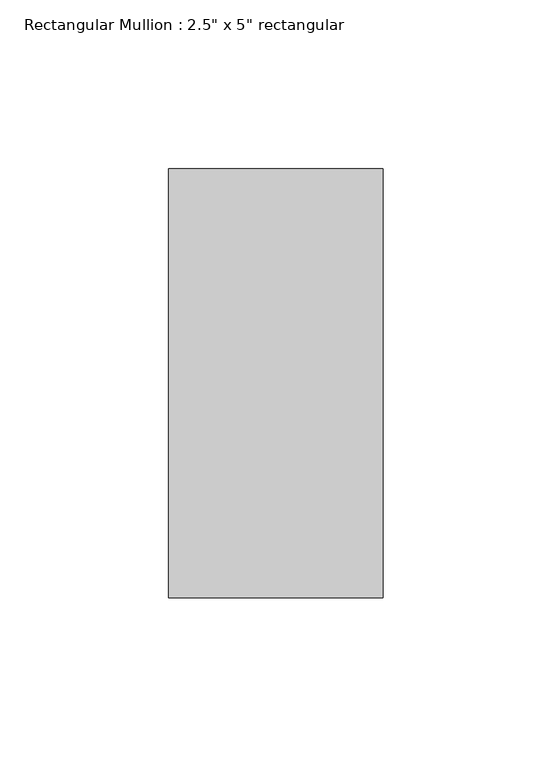
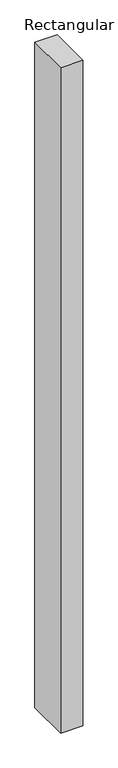
"""IFC4 building model written with IfcOpenShell, lengths in millimetres: member geometry."""

from ifc_helpers import new_model, si_unit, frame, origin, place, context, project, spatial, polyline, outline, extrude, source, transform, mapped, element, save


def member_9d47184b(model_context):
    return source(origin(), model_context, "Body", "SweptSolid", [
        extrude(outline(polyline([(31.75, 63.5), (31.75, -63.5), (-31.75, -63.5), (-31.75, 63.5), (31.75, 63.5)])), frame((0.0, 0.0, -2006.6), z_axis=(0.0, 0.0, 1.0), x_axis=(1.0, 0.0, 0.0)), (0.0, 0.0, 1.0), 2006.6),
    ])


if __name__ == "__main__":
    model = new_model("IFC4")
    model_context = context("Model", 3, world=origin())
    ifc_project = project(units=[si_unit("LENGTHUNIT", "METRE", prefix="MILLI")], contexts=[model_context])
    site = spatial("IfcSite", under=ifc_project)
    building = spatial("IfcBuilding", under=site)
    placement = place(None, origin())
    member_shape = member_9d47184b(model_context)
    element("IfcMember", 1, ObjectType="Rectangular Mullion : 2.5\" x 5\" rectangular", at=placement, inside=building, context=model_context, shape_type="MappedRepresentation", body=[
        mapped(member_shape, transform((0.0, 0.0, 0.0), x_axis=(1.0, 0.0, 0.0), y_axis=(0.0, 1.0, 0.0), z_axis=(0.0, 0.0, 1.0))),
    ])
    save(model, "model.ifc")

# Revit data of these elements
# Type "Rectangular Mullion : 2.5\" x 5\" rectangular"
#   built-in parameter 1007304 = 0.416667 (stored number, unit not read)
#   built-in parameter 1007301 = 0.104167 (stored number, unit not read)
#   built-in parameter 1007300 = 0.104167 (stored number, unit not read)
# Element 1 (IfcMember, "Rectangular Mullion : 2.5\" x 5\" rectangular")
#   Materials on its faces: "door black"
# Materials
#   "door black": class "Generic", colour RGB 120 120 120, transparency 0, Cost = 0
